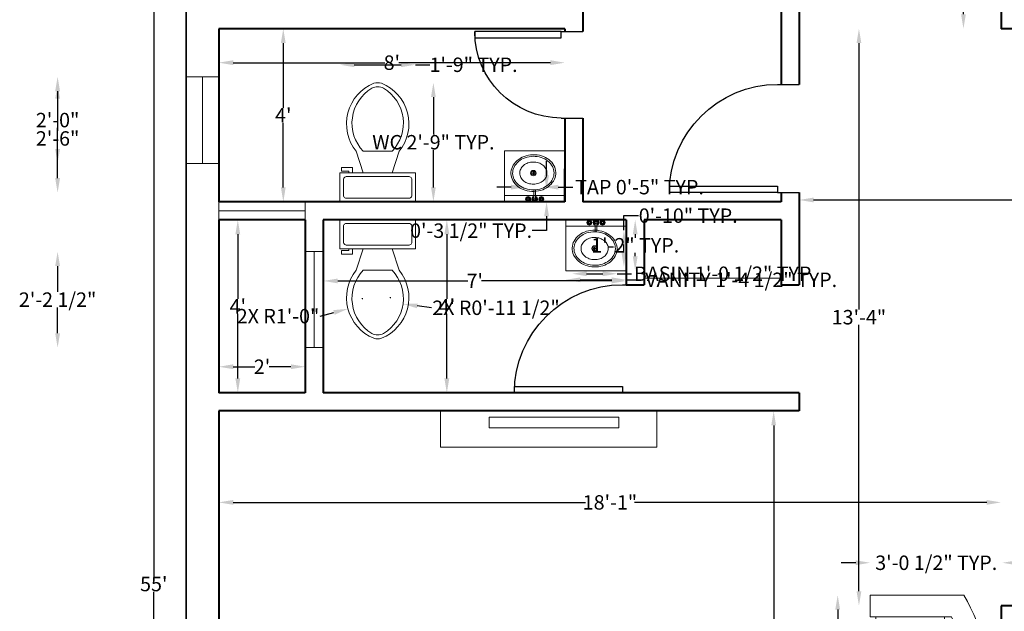
# Model space of a CAD drawing. Units: inches. Extents: x -46 to 447, y -42 to 702.
# Tile 4 of 7: x -46 to 227, y 322 to 487. Entities that reach past the tile are written whole.
import ezdxf

# ---------------------------------------------------------------- set-up
doc = ezdxf.new("R2010")
doc.units = ezdxf.units.IN
doc.header["$PDMODE"] = 3
for name, color, linetype, lineweight in [('A-ANNO-DIMS', 2, 'Continuous', 13), ('A-DOOR', 3, 'Continuous', 25), ('A-FLOR-CASE', 32, 'Continuous', 18), ('A-FLOR-FIXT', 9, 'Continuous', 20), ('A-FURN', 8, 'Continuous', 18), ('A-GLAZ', 4, 'Continuous', 18), ('A-WALL', 7, 'Continuous', 40), ('L-WALL', 7, 'Continuous', 35)]:
    doc.layers.add(name, color=color, linetype=linetype, lineweight=lineweight)
doc.styles.get("Standard").update_dxf_attribs({"font": 'arial.ttf'})
doc.dimstyles.get("Standard").update_dxf_attribs({"dimtxt": 4, "dimasz": 4, "dimexe": 0.18, "dimexo": 0.0625, "dimgap": 0.09, "dimtad": 0, "dimtih": 1, "dimtoh": 1, "dimdec": 0, "dimzin": 0, "dimdsep": 46, "dimlunit": 3, "dimtxsty": 'Standard', "dimcen": 0.09, "dimse1": 1, "dimse2": 1, "dimadec": 0, "dimazin": 0, "dimtfac": 1, "dimtdec": 0, "dimtofl": 0, "dimtmove": 0, "dimatfit": 3, "dimfxl": 1, "dimtolj": 1, "dimtzin": 0, "dimarcsym": 0})

# ---------------------------------------------------------------- blocks, each defined once
blk = doc.blocks.new('*U3')
for p, q in [((-30, 0), (-30, -6)), ((0, 0), (0, -6))]:
    blk.add_line(p, q)
blk.add_lwpolyline([(0, 0), (0, 30), (-1.75, 30), (-1.75, 0)], close=True)
blk.add_arc((0, 0), 30, 90, 180)
blk = doc.blocks.new('*U4')
for p, q in [((0, 0), (0, -6)), ((24, 0), (24, -6))]:
    blk.add_line(p, q)
blk.add_lwpolyline([(0, 0), (0, 24), (1.75, 24), (1.75, 0)], close=True)
blk.add_arc((0, 0), 24, 0, 90)
blk = doc.blocks.new('Faucet - Bathroom top')
for p, q in [((-4.107, 0.125), (-4.375, 0.125)), ((-3.75, 0.4788), (-3.75, 0.75)), ((-3.5, 0.482), (-3.5, 0.75)), ((-3.1461, 0.125), (-2.875, 0.125)), ((3.143, 0.125), (2.875, 0.125)), ((3.5, 0.4788), (3.5, 0.75)), ((3.75, 0.482), (3.75, 0.75)), ((4.1039, 0.125), (4.375, 0.125)), ((-4.1039, -0.125), (-4.375, -0.125)), ((-3.75, -0.4821), (-3.75, -0.75)), ((-3.5, -0.4789), (-3.5, -0.75)), ((-3.143, -0.125), (-2.875, -0.125)), ((-0.5, -0.8639), (-0.5, -4.5)), ((0.5, -4.5), (0.5, -0.8631)), ((3.1461, -0.125), (2.875, -0.125)), ((3.5, -0.4821), (3.5, -0.75)), ((3.75, -0.4789), (3.75, -0.75)), ((4.107, -0.125), (4.375, -0.125))]:
    blk.add_line(p, q)
for centre, radius in [((-3.625, 0), 1.375), ((-4.625, 0), 0.2795), ((-3.625, 0), 0.5), ((-3.625, 1), 0.2795), ((-2.625, 0), 0.2795), ((0, 0), 0.5), ((3.625, 0), 1.375), ((2.625, 0), 0.2795), ((3.625, 0), 0.5), ((3.625, 1), 0.2795), ((4.625, 0), 0.2795), ((-3.625, -1), 0.2795), ((3.625, -1), 0.2795)]:
    blk.add_circle(centre, radius)
for centre, radius, start, end in [((-3.625, 0), 1, 105.2407, 164.2093), ((-3.625, 0), 1, 16.44125, 74.07887), ((0, 0), 1.5, 289.6514, 250.3603), ((0, 0), 1, 300.3431, 239.7554), ((3.625, 0), 1, 106.12, 164.0884), ((3.625, 0), 1, 16.23422, 73.90469), ((-3.625, 0), 1, 196.2342, 253.9047), ((-3.625, 0), 1, 286.12, 344.0884), ((0, -4.5), 0.5, 180, 0), ((3.625, 0), 1, 196.4413, 254.0789), ((3.625, 0), 1, 285.2407, 344.2093)]:
    blk.add_arc(centre, radius, start, end)
blk = doc.blocks.new('Sink - Oval top')
for p, q in [((-1, 0), (1, 0)), ((0, 1), (0, -1))]:
    blk.add_line(p, q)
for points in [[(-12.23, 0.39, 0.117634), (-11.46, -3.36, 0.104469), (-8.88, -6.8, 0.090016), (-5.08, -9.07, 0.08192), (-0.32, -10.02, 0.08192), (4.49, -9.38, 0.090016), (8.42, -7.36, 0.104469), (11.22, -4.09, 0.117634), (12.23, -0.39, 0.117634), (11.46, 3.36, 0.104469), (8.88, 6.8, 0.090016), (5.08, 9.07, 0.08192), (0.32, 10.02, 0.08192), (-4.49, 9.38, 0.090016), (-8.42, 7.36, 0.104469), (-11.22, 4.09, 0.117634)], [(-11.29, 0.16, 0.118622), (-10.52, -3.25, 0.104678), (-8.07, -6.36, 0.089562), (-4.54, -8.37, 0.081185), (-0.13, -9.15, 0.081185), (4.3, -8.49, 0.089562), (7.89, -6.58, 0.104678), (10.42, -3.55, 0.118622), (11.29, -0.16, 0.118622), (10.52, 3.25, 0.104678), (8.07, 6.36, 0.089562), (4.54, 8.37, 0.081185), (0.13, 9.15, 0.081185), (-4.3, 8.49, 0.089562), (-7.89, 6.58, 0.104678), (-10.42, 3.55, 0.118622)], [(-7.42, 0.08, 0.118283), (-6.91, -2.17, 0.104607), (-5.29, -4.21, 0.089718), (-2.97, -5.53, 0.081436), (-0.07, -6.04, 0.081436), (2.84, -5.59, 0.089718), (5.2, -4.33, 0.104607), (6.86, -2.32, 0.118283), (7.42, -0.08, 0.118283), (6.91, 2.17, 0.104607), (5.29, 4.21, 0.089718), (2.97, 5.53, 0.081436), (0.07, 6.04, 0.081436), (-2.84, 5.59, 0.089718), (-5.2, 4.33, 0.104607), (-6.86, 2.32, 0.118283)]]:
    blk.add_lwpolyline(points, format="xyb", close=True)
for radius in [1.5, 1]:
    blk.add_circle((0, 0), radius)
blk = doc.blocks.new('Toilet - top')
for p, q in [((9.5, -6), (9.5, -2)), ((-8, -8.5), (-8, -8)), ((-7, -8), (-7, -9.5)), ((-4, -8), (-6, -14)), ((4, -8), (6, -14)), ((-10, -8.5), (-8, -8.5)), ((-10, -9.5), (-10, -8.5)), ((-7, -9.5), (-10, -9.5)), ((4, -14), (-4, -14))]:
    blk.add_line(p, q)
blk.add_lwpolyline([(10.5, -8), (10.5, 0), (-10.5, 0), (-10.5, -8)], close=True)
for points in [[(-9.5, -2), (-9.5, -6)], [(8.5, -1), (-8.5, -1)], [(-8.5, -7), (8.5, -7)]]:
    blk.add_lwpolyline(points)
for centre, radius, start, end in [((-8.62, -1.88), 0.884, 81.8699, 188.1301), ((8.62, -1.88), 0.884, 351.8699, 98.1301), ((-8.62, -6.12), 0.884, 171.8699, 278.1301), ((8.62, -6.12), 0.884, 261.8699, 8.1301), ((3.52, -21.58), 12.17, 141.4691, 247.9714), ((4.2, -21.82), 11.33, 136.3677, 238.9468), ((-3.52, -21.58), 12.17, 292.0284, 38.5307), ((-4.2, -21.82), 11.33, 301.053, 43.6321), ((0, -27.88), 4, 245.7318, 294.2682), ((0, -29), 4, 254.8605, 285.1395)]:
    blk.add_arc(centre, radius, start, end)
blk = doc.blocks.new('Sofa - Roundback Loveseat 5 ft.')
for p, q in [((0, -32.44198), (0, -5.99998)), ((-24, -33.99998), (-24, -11.46958)), ((-23.9998, -13.38178), (23.99986, -13.38178)), ((24.00004, -33.99998), (24.00004, -11.46958)), ((-24, -32.44198), (24.00004, -32.44198))]:
    blk.add_line(p, q)
for points in [[(-24, -33.99998), (-30, -33.99998), (-30, -7.99998)], [(30.00004, -7.99998), (30.00004, -33.99998), (24.00004, -33.99998)]]:
    blk.add_lwpolyline(points)
for centre, radius, start, end in [((0, -60.24998), 60.24998, 60.13715, 119.8628), ((0, -61.38438), 55.38444, 64.32083, 115.6792)]:
    blk.add_arc(centre, radius, start, end)
blk = doc.blocks.new('*D50')
at = {"layer": 'A-ANNO-DIMS', "color": 0, "lineweight": -2, "transparency": 16777216}
for p, q in [((-9.03, 656), (-9.03, 332.12)), ((-9.03, 4), (-9.03, 327.88))]:
    blk.add_line(p, q, dxfattribs=at)
at = {"layer": 'A-ANNO-DIMS', "color": 0, "transparency": 16777216}
for points in [[(-9.7, 656), (-8.36, 656), (-9.03, 660)], [(-9.7, 4), (-8.36, 4), (-9.03, 0)]]:
    blk.add_solid(points, dxfattribs=at)
at = {"layer": 'Defpoints', "color": 0, "transparency": 16777216}
for p in [(0, 660), (0, 0), (-9.03, 0)]:
    blk.add_point(p, dxfattribs=at)
at = {"layer": 'A-ANNO-DIMS', "color": 0, "transparency": 16777216, "insert": (-9.03, 330), "char_height": 4, "attachment_point": 5}
blk.add_mtext("\\A1;55'", dxfattribs=at)
blk = doc.blocks.new('*D61')
at = {"layer": 'A-ANNO-DIMS', "color": 0, "lineweight": -2, "transparency": 16777216}
for p, q in [((174, 436.51), (250.67, 436.51)), ((344, 436.51), (267.33, 436.51))]:
    blk.add_line(p, q, dxfattribs=at)
at = {"layer": 'A-ANNO-DIMS', "color": 0, "transparency": 16777216}
for points in [[(174, 437.18), (174, 435.84), (170, 436.51)], [(344, 437.18), (344, 435.84), (348, 436.51)]]:
    blk.add_solid(points, dxfattribs=at)
at = {"layer": 'Defpoints', "color": 0, "transparency": 16777216}
for p in [(170, 468.57), (348, 468.57), (348, 436.51)]:
    blk.add_point(p, dxfattribs=at)
at = {"layer": 'A-ANNO-DIMS', "color": 0, "transparency": 16777216, "insert": (259, 436.51), "char_height": 4, "attachment_point": 5}
blk.add_mtext('\\A1;14\'-10"', dxfattribs=at)
blk = doc.blocks.new('*D62')
at = {"layer": 'A-ANNO-DIMS', "color": 0, "lineweight": -2, "transparency": 16777216}
for p, q in [((186.57, 480), (186.57, 406.13)), ((186.57, 328), (186.57, 401.87))]:
    blk.add_line(p, q, dxfattribs=at)
at = {"layer": 'A-ANNO-DIMS', "color": 0, "transparency": 16777216}
for points in [[(185.91, 480), (187.24, 480), (186.57, 484)], [(185.91, 328), (187.24, 328), (186.57, 324)]]:
    blk.add_solid(points, dxfattribs=at)
at = {"layer": 'Defpoints', "color": 0, "transparency": 16777216}
for p in [(312.89, 484), (186.57, 324), (312.89, 324)]:
    blk.add_point(p, dxfattribs=at)
at = {"layer": 'A-ANNO-DIMS', "color": 0, "transparency": 16777216, "insert": (186.57, 404), "char_height": 4, "attachment_point": 5}
blk.add_mtext('\\A1;13\'-4"', dxfattribs=at)
blk = doc.blocks.new('*D63')
at = {"layer": 'A-ANNO-DIMS', "color": 0, "lineweight": -2, "transparency": 16777216}
for p, q in [((13, 352.64), (110.73, 352.64)), ((222, 352.64), (124.27, 352.64))]:
    blk.add_line(p, q, dxfattribs=at)
at = {"layer": 'A-ANNO-DIMS', "color": 0, "transparency": 16777216}
for points in [[(13, 353.31), (13, 351.98), (9, 352.64)], [(222, 353.31), (222, 351.98), (226, 352.64)]]:
    blk.add_solid(points, dxfattribs=at)
at = {"layer": 'Defpoints', "color": 0, "transparency": 16777216}
for p in [(9, 352.64), (9, 324), (226, 324)]:
    blk.add_point(p, dxfattribs=at)
at = {"layer": 'A-ANNO-DIMS', "color": 0, "transparency": 16777216, "insert": (117.5, 352.64), "char_height": 4, "attachment_point": 5}
blk.add_mtext('\\A1;18\'-1"', dxfattribs=at)
blk = doc.blocks.new('*D64')
at = {"layer": 'A-ANNO-DIMS', "color": 0, "lineweight": -2, "transparency": 16777216}
for p, q in [((162.92, 374), (162.92, 296.1)), ((162.92, 214), (162.92, 291.9))]:
    blk.add_line(p, q, dxfattribs=at)
at = {"layer": 'A-ANNO-DIMS', "color": 0, "transparency": 16777216}
for points in [[(162.25, 374), (163.58, 374), (162.92, 378)], [(162.25, 214), (163.58, 214), (162.92, 210)]]:
    blk.add_solid(points, dxfattribs=at)
at = {"layer": 'Defpoints', "color": 0, "transparency": 16777216}
for p in [(9, 378), (9, 210), (162.92, 210)]:
    blk.add_point(p, dxfattribs=at)
at = {"layer": 'A-ANNO-DIMS', "color": 0, "transparency": 16777216, "insert": (162.92, 294), "char_height": 4, "attachment_point": 5}
blk.add_mtext("\\A1;14'", dxfattribs=at)
blk = doc.blocks.new('*D65')
at = {"layer": 'A-ANNO-DIMS', "color": 0, "lineweight": -2, "transparency": 16777216}
for p, q in [((14.28, 427), (14.28, 409.09)), ((14.28, 387), (14.28, 404.91))]:
    blk.add_line(p, q, dxfattribs=at)
at = {"layer": 'A-ANNO-DIMS', "color": 0, "transparency": 16777216}
for points in [[(13.61, 427), (14.95, 427), (14.28, 431)], [(13.61, 387), (14.95, 387), (14.28, 383)]]:
    blk.add_solid(points, dxfattribs=at)
at = {"layer": 'Defpoints', "color": 0, "transparency": 16777216}
for p in [(9, 431), (9, 383), (14.28, 383)]:
    blk.add_point(p, dxfattribs=at)
at = {"layer": 'A-ANNO-DIMS', "color": 0, "transparency": 16777216, "insert": (14.28, 407), "char_height": 4, "attachment_point": 5}
blk.add_mtext("\\A1;4'", dxfattribs=at)
blk = doc.blocks.new('*D66')
at = {"layer": 'A-ANNO-DIMS', "color": 0, "lineweight": -2, "transparency": 16777216}
for p, q in [((13, 390.26), (19.04, 390.26)), ((29, 390.26), (22.96, 390.26))]:
    blk.add_line(p, q, dxfattribs=at)
at = {"layer": 'A-ANNO-DIMS', "color": 0, "transparency": 16777216}
for points in [[(13, 390.93), (13, 389.6), (9, 390.26)], [(29, 390.93), (29, 389.6), (33, 390.26)]]:
    blk.add_solid(points, dxfattribs=at)
at = {"layer": 'Defpoints', "color": 0, "transparency": 16777216}
for p in [(9, 390.26), (9, 383), (33, 383)]:
    blk.add_point(p, dxfattribs=at)
at = {"layer": 'A-ANNO-DIMS', "color": 0, "transparency": 16777216, "insert": (21, 390.26), "char_height": 4, "attachment_point": 5}
blk.add_mtext("\\A1;2'", dxfattribs=at)
blk = doc.blocks.new('*D67')
at = {"layer": 'A-ANNO-DIMS', "color": 0, "lineweight": -2, "transparency": 16777216}
for p, q in [((42, 414.06), (78.09, 414.06)), ((118, 414.06), (81.91, 414.06))]:
    blk.add_line(p, q, dxfattribs=at)
at = {"layer": 'A-ANNO-DIMS', "color": 0, "transparency": 16777216}
for points in [[(42, 414.72), (42, 413.39), (38, 414.06)], [(118, 414.72), (118, 413.39), (122, 414.06)]]:
    blk.add_solid(points, dxfattribs=at)
at = {"layer": 'Defpoints', "color": 0, "transparency": 16777216}
for p in [(38, 431), (122, 431), (38, 414.06)]:
    blk.add_point(p, dxfattribs=at)
at = {"layer": 'A-ANNO-DIMS', "color": 0, "transparency": 16777216, "insert": (80, 414.06), "char_height": 4, "attachment_point": 5}
blk.add_mtext("\\A1;7'", dxfattribs=at)
blk = doc.blocks.new('*D68')
at = {"layer": 'A-ANNO-DIMS', "color": 0, "lineweight": -2, "transparency": 16777216}
for p, q in [((72.26, 427), (72.26, 409.09)), ((72.26, 387), (72.26, 404.91))]:
    blk.add_line(p, q, dxfattribs=at)
at = {"layer": 'A-ANNO-DIMS', "color": 0, "transparency": 16777216}
for points in [[(71.59, 427), (72.93, 427), (72.26, 431)], [(71.59, 387), (72.93, 387), (72.26, 383)]]:
    blk.add_solid(points, dxfattribs=at)
at = {"layer": 'Defpoints', "color": 0, "transparency": 16777216}
for p in [(38, 431), (38, 383), (72.26, 383)]:
    blk.add_point(p, dxfattribs=at)
at = {"layer": 'A-ANNO-DIMS', "color": 0, "transparency": 16777216, "insert": (72.26, 407), "char_height": 4, "attachment_point": 5}
blk.add_mtext("\\A1;4'", dxfattribs=at)
blk = doc.blocks.new('*D69')
at = {"layer": 'A-ANNO-DIMS', "color": 0, "lineweight": -2, "transparency": 16777216}
for p, q in [((215.55, 546), (215.55, 519.13)), ((215.55, 488), (215.55, 514.87))]:
    blk.add_line(p, q, dxfattribs=at)
at = {"layer": 'A-ANNO-DIMS', "color": 0, "transparency": 16777216}
for points in [[(214.89, 546), (216.22, 546), (215.55, 550)], [(214.89, 488), (216.22, 488), (215.55, 484)]]:
    blk.add_solid(points, dxfattribs=at)
at = {"layer": 'Defpoints', "color": 0, "transparency": 16777216}
for p in [(226, 550), (215.55, 484), (226, 484)]:
    blk.add_point(p, dxfattribs=at)
at = {"layer": 'A-ANNO-DIMS', "color": 0, "transparency": 16777216, "insert": (215.55, 517), "char_height": 4, "attachment_point": 5}
blk.add_mtext('\\A1;5\'-6"', dxfattribs=at)
blk = doc.blocks.new('*D75')
at = {"layer": 'A-ANNO-DIMS', "color": 0, "lineweight": -2, "transparency": 16777216}
for p, q in [((13, 474.58), (55.07, 474.58)), ((101, 474.58), (58.93, 474.58))]:
    blk.add_line(p, q, dxfattribs=at)
at = {"layer": 'A-ANNO-DIMS', "color": 0, "transparency": 16777216}
for points in [[(13, 475.25), (13, 473.92), (9, 474.58)], [(101, 475.25), (101, 473.92), (105, 474.58)]]:
    blk.add_solid(points, dxfattribs=at)
at = {"layer": 'Defpoints', "color": 0, "transparency": 16777216}
for p in [(9, 484), (105, 484), (9, 474.58)]:
    blk.add_point(p, dxfattribs=at)
at = {"layer": 'A-ANNO-DIMS', "color": 0, "transparency": 16777216, "insert": (57, 474.58), "char_height": 4, "attachment_point": 5}
blk.add_mtext("\\A1;8'", dxfattribs=at)
blk = doc.blocks.new('*D76')
at = {"layer": 'A-ANNO-DIMS', "color": 0, "lineweight": -2, "transparency": 16777216}
for p, q in [((26.9, 480), (26.9, 462.09)), ((26.9, 440), (26.9, 457.91))]:
    blk.add_line(p, q, dxfattribs=at)
at = {"layer": 'A-ANNO-DIMS', "color": 0, "transparency": 16777216}
for points in [[(26.23, 480), (27.56, 480), (26.9, 484)], [(26.23, 440), (27.56, 440), (26.9, 436)]]:
    blk.add_solid(points, dxfattribs=at)
at = {"layer": 'Defpoints', "color": 0, "transparency": 16777216}
for p in [(9, 484), (9, 436), (26.9, 436)]:
    blk.add_point(p, dxfattribs=at)
at = {"layer": 'A-ANNO-DIMS', "color": 0, "transparency": 16777216, "insert": (26.9, 460), "char_height": 4, "attachment_point": 5}
blk.add_mtext("\\A1;4'", dxfattribs=at)
blk = doc.blocks.new('VANITY-TOP')
for points in [[(0, -1.75), (16.74, -1.75), (16.74, 0), (0, 0)], [(0, -1.75), (16.74, -1.75), (16.74, -14.12), (0, -14.12)]]:
    blk.add_lwpolyline(points, close=True)
blk = doc.blocks.new('*D94')
at = {"layer": 'A-ANNO-DIMS', "color": 0, "lineweight": -2, "transparency": 16777216}
for p, q in [((90.09, 440.07), (86.09, 440.07)), ((103.17, 440.07), (107.17, 440.07))]:
    blk.add_line(p, q, dxfattribs=at)
at = {"layer": 'A-ANNO-DIMS', "color": 0, "transparency": 16777216}
for points in [[(90.09, 440.74), (90.09, 439.4), (94.09, 440.07)], [(103.17, 440.74), (103.17, 439.4), (99.17, 440.07)]]:
    blk.add_solid(points, dxfattribs=at)
at = {"layer": 'Defpoints', "color": 0, "transparency": 16777216}
for p in [(99.17, 440.07), (94.09, 439.31), (99.17, 439.31)]:
    blk.add_point(p, dxfattribs=at)
at = {"layer": 'A-ANNO-DIMS', "color": 0, "transparency": 16777216, "insert": (125.71, 440.07), "char_height": 4, "attachment_point": 5}
blk.add_mtext('\\A1;TAP 0\'-5" TYP.', dxfattribs=at)
blk = doc.blocks.new('*D95')
at = {"layer": 'A-ANNO-DIMS', "color": 0, "lineweight": -2, "transparency": 16777216}
for p, q in [((99.93, 443.31), (99.93, 447.31)), ((99.93, 432), (99.93, 428)), ((99.93, 428), (95.93, 428))]:
    blk.add_line(p, q, dxfattribs=at)
at = {"layer": 'A-ANNO-DIMS', "color": 0, "transparency": 16777216}
for points in [[(99.27, 443.31), (100.6, 443.31), (99.93, 439.31)], [(99.27, 432), (100.6, 432), (99.93, 436)]]:
    blk.add_solid(points, dxfattribs=at)
at = {"layer": 'Defpoints', "color": 0, "transparency": 16777216}
for p in [(99.17, 439.31), (99.17, 436), (99.93, 436)]:
    blk.add_point(p, dxfattribs=at)
at = {"layer": 'A-ANNO-DIMS', "color": 0, "transparency": 16777216, "insert": (78.99, 428), "char_height": 4, "attachment_point": 5}
blk.add_mtext('\\A1;0\'-3 1/2" TYP.', dxfattribs=at)
blk = doc.blocks.new('*D96')
at = {"layer": 'A-ANNO-DIMS', "color": 0, "lineweight": -2, "transparency": 16777216}
for p, q in [((111.02, 416.05), (115.51, 416.05)), ((119.51, 416.05), (123.51, 416.05))]:
    blk.add_line(p, q, dxfattribs=at)
at = {"layer": 'A-ANNO-DIMS', "color": 0, "transparency": 16777216}
for points in [[(111.02, 416.72), (111.02, 415.38), (107.02, 416.05)], [(115.51, 416.72), (115.51, 415.38), (119.51, 416.05)]]:
    blk.add_solid(points, dxfattribs=at)
at = {"layer": 'Defpoints', "color": 0, "transparency": 16777216}
for p in [(107.02, 417.92), (119.51, 417.92), (119.51, 416.05)]:
    blk.add_point(p, dxfattribs=at)
at = {"layer": 'A-ANNO-DIMS', "color": 0, "transparency": 16777216, "insert": (149.52, 416.05), "char_height": 4, "attachment_point": 5}
blk.add_mtext('\\A1;BASIN 1\'-0 1/2" TYP.', dxfattribs=at)
blk = doc.blocks.new('*D97')
at = {"layer": 'A-ANNO-DIMS', "color": 0, "lineweight": -2, "transparency": 16777216}
for p, q in [((121.38, 428.16), (121.38, 432.16)), ((121.38, 432.16), (125.38, 432.16)), ((121.38, 421.92), (121.38, 424.16))]:
    blk.add_line(p, q, dxfattribs=at)
at = {"layer": 'A-ANNO-DIMS', "color": 0, "transparency": 16777216}
for points in [[(120.71, 424.16), (122.04, 424.16), (121.38, 428.16)], [(120.71, 421.92), (122.04, 421.92), (121.38, 417.92)]]:
    blk.add_solid(points, dxfattribs=at)
at = {"layer": 'Defpoints', "color": 0, "transparency": 16777216}
for p in [(119.51, 428.16), (121.38, 428.16), (119.51, 417.92)]:
    blk.add_point(p, dxfattribs=at)
at = {"layer": 'A-ANNO-DIMS', "color": 0, "transparency": 16777216, "insert": (139.21, 432.16), "char_height": 4, "attachment_point": 5}
blk.add_mtext('\\A1;0\'-10" TYP.', dxfattribs=at)
blk = doc.blocks.new('*D98')
at = {"layer": 'A-ANNO-DIMS', "color": 0, "lineweight": -2, "transparency": 16777216}
for p, q in [((68.53, 465.05), (68.53, 454.68)), ((68.53, 440), (68.53, 450.36))]:
    blk.add_line(p, q, dxfattribs=at)
at = {"layer": 'A-ANNO-DIMS', "color": 0, "transparency": 16777216}
for points in [[(67.87, 465.05), (69.2, 465.05), (68.53, 469.05)], [(67.87, 440), (69.2, 440), (68.53, 436)]]:
    blk.add_solid(points, dxfattribs=at)
at = {"layer": 'Defpoints', "color": 0, "transparency": 16777216}
for p in [(63.58, 469.05), (63.58, 436), (68.53, 436)]:
    blk.add_point(p, dxfattribs=at)
at = {"layer": 'A-ANNO-DIMS', "color": 0, "transparency": 16777216, "insert": (68.53, 452.52), "char_height": 4, "attachment_point": 5}
blk.add_mtext('\\A1;WC 2\'-9" TYP.', dxfattribs=at)
blk = doc.blocks.new('*D99')
at = {"layer": 'A-ANNO-DIMS', "color": 0, "lineweight": -2, "transparency": 16777216}
for p, q in [((46.58, 474), (59.58, 474)), ((63.58, 474), (67.58, 474))]:
    blk.add_line(p, q, dxfattribs=at)
at = {"layer": 'A-ANNO-DIMS', "color": 0, "transparency": 16777216}
for points in [[(46.58, 474.67), (46.58, 473.34), (42.58, 474)], [(59.58, 474.67), (59.58, 473.34), (63.58, 474)]]:
    blk.add_solid(points, dxfattribs=at)
at = {"layer": 'Defpoints', "color": 0, "transparency": 16777216}
for p in [(63.58, 474), (42.58, 469.05), (63.58, 469.05)]:
    blk.add_point(p, dxfattribs=at)
at = {"layer": 'A-ANNO-DIMS', "color": 0, "transparency": 16777216, "insert": (79.67, 474), "char_height": 4, "attachment_point": 5}
blk.add_mtext('\\A1;1\'-9" TYP.', dxfattribs=at)
blk = doc.blocks.new('*D100')
at = {"layer": 'A-ANNO-DIMS', "color": 0, "lineweight": -2, "transparency": 16777216}
for p, q in [((109.26, 414.37), (118, 414.37)), ((122, 414.37), (126, 414.37))]:
    blk.add_line(p, q, dxfattribs=at)
at = {"layer": 'A-ANNO-DIMS', "color": 0, "transparency": 16777216}
for points in [[(109.26, 415.03), (109.26, 413.7), (105.26, 414.37)], [(118, 415.03), (118, 413.7), (122, 414.37)]]:
    blk.add_solid(points, dxfattribs=at)
at = {"layer": 'Defpoints', "color": 0, "transparency": 16777216}
for p in [(105.26, 416.88), (122, 416.88), (122, 414.37)]:
    blk.add_point(p, dxfattribs=at)
at = {"layer": 'A-ANNO-DIMS', "color": 0, "transparency": 16777216, "insert": (153.91, 414.37), "char_height": 4, "attachment_point": 5}
blk.add_mtext('\\A1;VANITY 1\'-4 1/2" TYP.', dxfattribs=at)
blk = doc.blocks.new('*D101')
at = {"layer": 'A-ANNO-DIMS', "color": 0, "lineweight": -2, "transparency": 16777216}
for p, q in [((124.51, 427), (124.51, 426.04)), ((124.51, 420.88), (124.51, 421.84))]:
    blk.add_line(p, q, dxfattribs=at)
at = {"layer": 'A-ANNO-DIMS', "color": 0, "transparency": 16777216}
for points in [[(123.84, 427), (125.18, 427), (124.51, 431)], [(123.84, 420.88), (125.18, 420.88), (124.51, 416.88)]]:
    blk.add_solid(points, dxfattribs=at)
at = {"layer": 'Defpoints', "color": 0, "transparency": 16777216}
for p in [(122, 431), (124.51, 431), (122, 416.88)]:
    blk.add_point(p, dxfattribs=at)
at = {"layer": 'A-ANNO-DIMS', "color": 0, "transparency": 16777216, "insert": (124.51, 423.94), "char_height": 4, "attachment_point": 5}
blk.add_mtext('\\A1;1\'-2" TYP.', dxfattribs=at)
blk = doc.blocks.new('*D106')
at = {"layer": 'A-ANNO-DIMS', "color": 0, "lineweight": -2, "transparency": 16777216}
for p, q in [((180.68, 322.9), (180.68, 299.06)), ((180.68, 270.9), (180.68, 294.74))]:
    blk.add_line(p, q, dxfattribs=at)
at = {"layer": 'A-ANNO-DIMS', "color": 0, "transparency": 16777216}
for points in [[(180.01, 322.9), (181.34, 322.9), (180.68, 326.9)], [(180.01, 270.9), (181.34, 270.9), (180.68, 266.9)]]:
    blk.add_solid(points, dxfattribs=at)
at = {"layer": 'Defpoints', "color": 0, "transparency": 16777216}
for p in [(180.68, 326.9), (189.68, 326.9), (189.68, 266.9)]:
    blk.add_point(p, dxfattribs=at)
at = {"layer": 'A-ANNO-DIMS', "color": 0, "transparency": 16777216, "insert": (180.68, 296.9), "char_height": 4, "attachment_point": 5}
blk.add_mtext('\\A1;LOVESEAT 5\'-0" TYP.', dxfattribs=at)
blk = doc.blocks.new('*D107')
at = {"layer": 'A-ANNO-DIMS', "color": 0, "lineweight": -2, "transparency": 16777216}
for p, q in [((185.68, 335.9), (181.68, 335.9)), ((230.34, 335.9), (234.34, 335.9))]:
    blk.add_line(p, q, dxfattribs=at)
at = {"layer": 'A-ANNO-DIMS', "color": 0, "transparency": 16777216}
for points in [[(185.68, 336.57), (185.68, 335.24), (189.68, 335.9)], [(230.34, 336.57), (230.34, 335.24), (226.34, 335.9)]]:
    blk.add_solid(points, dxfattribs=at)
at = {"layer": 'Defpoints', "color": 0, "transparency": 16777216}
for p in [(226.34, 335.9), (189.68, 326.9), (226.34, 326.9)]:
    blk.add_point(p, dxfattribs=at)
at = {"layer": 'A-ANNO-DIMS', "color": 0, "transparency": 16777216, "insert": (208.01, 335.9), "char_height": 4, "attachment_point": 5}
blk.add_mtext('\\A1;3\'-0 1/2" TYP.', dxfattribs=at)
blk = doc.blocks.new('*D125')
at = {"layer": 'A-ANNO-DIMS', "color": 0, "lineweight": -2, "transparency": 16777216}
for p, q in [((-35.7, 464.57), (-35.7, 455.71)), ((-35.7, 442.57), (-35.7, 451.44))]:
    blk.add_line(p, q, dxfattribs=at)
at = {"layer": 'A-ANNO-DIMS', "color": 0, "transparency": 16777216}
for points in [[(-36.37, 464.57), (-35.03, 464.57), (-35.7, 468.57)], [(-36.37, 442.57), (-35.03, 442.57), (-35.7, 438.57)]]:
    blk.add_solid(points, dxfattribs=at)
at = {"layer": 'Defpoints', "color": 0, "transparency": 16777216}
for p in [(-35.7, 468.57), (165, 468.57), (165, 438.57)]:
    blk.add_point(p, dxfattribs=at)
at = {"layer": 'A-ANNO-DIMS', "color": 0, "transparency": 16777216, "insert": (-35.7, 453.57), "char_height": 4, "attachment_point": 5}
blk.add_mtext('\\A1;2\'-6"', dxfattribs=at)
blk = doc.blocks.new('*D126')
at = {"layer": 'A-ANNO-DIMS', "color": 0, "lineweight": -2, "transparency": 16777216}
for p, q in [((431.7, 409), (431.7, 400.13)), ((431.7, 387), (431.7, 395.87))]:
    blk.add_line(p, q, dxfattribs=at)
at = {"layer": 'A-ANNO-DIMS', "color": 0, "transparency": 16777216}
for points in [[(431.03, 409), (432.37, 409), (431.7, 413)], [(431.03, 387), (432.37, 387), (431.7, 383)]]:
    blk.add_solid(points, dxfattribs=at)
at = {"layer": 'Defpoints', "color": 0, "transparency": 16777216}
for p in [(122, 413), (431.7, 413), (122.75, 383)]:
    blk.add_point(p, dxfattribs=at)
at = {"layer": 'A-ANNO-DIMS', "color": 0, "transparency": 16777216, "insert": (431.7, 398), "char_height": 4, "attachment_point": 5}
blk.add_mtext('\\A1;2\'-6"', dxfattribs=at)
blk = doc.blocks.new('*D127')
at = {"layer": 'A-ANNO-DIMS', "color": 0, "lineweight": -2, "transparency": 16777216}
for p, q in [((431.7, 479.23), (431.7, 473.36)), ((431.7, 463.23), (431.7, 469.1))]:
    blk.add_line(p, q, dxfattribs=at)
at = {"layer": 'A-ANNO-DIMS', "color": 0, "transparency": 16777216}
for points in [[(431.03, 479.23), (432.37, 479.23), (431.7, 483.23)], [(431.03, 463.23), (432.37, 463.23), (431.7, 459.23)]]:
    blk.add_solid(points, dxfattribs=at)
at = {"layer": 'Defpoints', "color": 0, "transparency": 16777216}
for p in [(105, 483.23), (431.7, 483.23), (105, 459.23)]:
    blk.add_point(p, dxfattribs=at)
at = {"layer": 'A-ANNO-DIMS', "color": 0, "transparency": 16777216, "insert": (431.7, 471.23), "char_height": 4, "attachment_point": 5}
blk.add_mtext('\\A1;2\'-0"', dxfattribs=at)
blk = doc.blocks.new('*D128')
at = {"layer": 'A-ANNO-DIMS', "color": 0, "lineweight": -2, "transparency": 16777216}
for p, q in [((-35.7, 466.66), (-35.7, 460.79)), ((-35.7, 450.66), (-35.7, 456.52))]:
    blk.add_line(p, q, dxfattribs=at)
at = {"layer": 'A-ANNO-DIMS', "color": 0, "transparency": 16777216}
for points in [[(-36.37, 466.66), (-35.03, 466.66), (-35.7, 470.66)], [(-36.37, 450.66), (-35.03, 450.66), (-35.7, 446.66)]]:
    blk.add_solid(points, dxfattribs=at)
at = {"layer": 'Defpoints', "color": 0, "transparency": 16777216}
for p in [(-35.7, 470.66), (0, 470.66), (0, 446.66)]:
    blk.add_point(p, dxfattribs=at)
at = {"layer": 'A-ANNO-DIMS', "color": 0, "transparency": 16777216, "insert": (-35.7, 458.66), "char_height": 4, "attachment_point": 5}
blk.add_mtext('\\A1;2\'-0"', dxfattribs=at)
blk = doc.blocks.new('*D129')
at = {"layer": 'A-ANNO-DIMS', "color": 0, "lineweight": -2, "transparency": 16777216}
for p, q in [((29, -35.7), (25, -35.7)), ((42, -35.7), (46, -35.7))]:
    blk.add_line(p, q, dxfattribs=at)
at = {"layer": 'A-ANNO-DIMS', "color": 0, "transparency": 16777216}
for points in [[(29, -35.03), (29, -36.37), (33, -35.7)], [(42, -35.03), (42, -36.37), (38, -35.7)]]:
    blk.add_solid(points, dxfattribs=at)
at = {"layer": 'Defpoints', "color": 0, "transparency": 16777216}
for p in [(33, 383), (38, 383), (38, -35.7)]:
    blk.add_point(p, dxfattribs=at)
at = {"layer": 'A-ANNO-DIMS', "color": 0, "transparency": 16777216, "insert": (51.41, -35.7), "char_height": 4, "attachment_point": 5}
blk.add_mtext('\\A1;0\'-5"', dxfattribs=at)
blk = doc.blocks.new('*D130')
at = {"layer": 'A-ANNO-DIMS', "color": 0, "lineweight": -2, "transparency": 16777216}
for p, q in [((0, 695.7), (-4, 695.7)), ((5, 695.7), (4, 695.7))]:
    blk.add_line(p, q, dxfattribs=at)
at = {"layer": 'A-ANNO-DIMS', "color": 0, "transparency": 16777216}
for points in [[(4, 696.37), (4, 695.03), (0, 695.7)], [(5, 696.37), (5, 695.03), (9, 695.7)]]:
    blk.add_solid(points, dxfattribs=at)
at = {"layer": 'Defpoints', "color": 0, "transparency": 16777216}
for p in [(0, 695.7), (0, 446.66), (9, 446.66)]:
    blk.add_point(p, dxfattribs=at)
at = {"layer": 'A-ANNO-DIMS', "color": 0, "transparency": 16777216, "insert": (-9.41, 695.7), "char_height": 4, "attachment_point": 5}
blk.add_mtext('\\A1;0\'-9"', dxfattribs=at)
blk = doc.blocks.new('*D138')
at = {"layer": 'A-ANNO-DIMS', "color": 0, "lineweight": -2, "transparency": 16777216}
for p, q in [((-35.7, 418.18), (-35.7, 411.03)), ((-35.7, 399.56), (-35.7, 406.71))]:
    blk.add_line(p, q, dxfattribs=at)
at = {"layer": 'A-ANNO-DIMS', "color": 0, "transparency": 16777216}
for points in [[(-36.37, 418.18), (-35.03, 418.18), (-35.7, 422.18)], [(-36.37, 399.56), (-35.03, 399.56), (-35.7, 395.56)]]:
    blk.add_solid(points, dxfattribs=at)
at = {"layer": 'Defpoints', "color": 0, "transparency": 16777216}
for p in [(-35.7, 422.18), (33, 422.18), (33, 395.56)]:
    blk.add_point(p, dxfattribs=at)
at = {"layer": 'A-ANNO-DIMS', "color": 0, "transparency": 16777216, "insert": (-35.7, 408.87), "char_height": 4, "attachment_point": 5}
blk.add_mtext('\\A1;2\'-2 1/2"', dxfattribs=at)
blk = doc.blocks.new('*D148')
at = {"layer": 'A-ANNO-DIMS', "color": 0, "lineweight": -2, "transparency": 16777216}
for p, q in [((227, 695.7), (223, 695.7)), ((238.24, 695.7), (242.24, 695.7))]:
    blk.add_line(p, q, dxfattribs=at)
at = {"layer": 'A-ANNO-DIMS', "color": 0, "transparency": 16777216}
for points in [[(227, 696.37), (227, 695.03), (231, 695.7)], [(238.24, 696.37), (238.24, 695.03), (234.24, 695.7)]]:
    blk.add_solid(points, dxfattribs=at)
at = {"layer": 'Defpoints', "color": 0, "transparency": 16777216}
for p in [(234.24, 695.7), (231, 319), (234.24, 319)]:
    blk.add_point(p, dxfattribs=at)
at = {"layer": 'A-ANNO-DIMS', "color": 0, "transparency": 16777216, "insert": (247.64, 695.7), "char_height": 4, "attachment_point": 5}
blk.add_mtext('\\A1;0\'-3"', dxfattribs=at)
blk = doc.blocks.new('*D159')
at = {"layer": 'A-ANNO-DIMS', "color": 0, "lineweight": -2, "transparency": 16777216}
for p, q in [((56.51, 409.42), (56.69, 409.42)), ((56.6, 409.33), (56.6, 409.51)), ((37.09, 404.29), (40.96, 405.31))]:
    blk.add_line(p, q, dxfattribs=at)
at = {"layer": 'A-ANNO-DIMS', "color": 0, "transparency": 16777216}
blk.add_solid([(40.79, 405.96), (41.13, 404.67), (44.83, 406.33)], dxfattribs=at)
at = {"layer": 'Defpoints', "color": 0, "transparency": 16777216}
for p in [(56.6, 409.42), (44.83, 406.33)]:
    blk.add_point(p, dxfattribs=at)
at = {"layer": 'A-ANNO-DIMS', "color": 0, "transparency": 16777216, "insert": (25.44, 404.29), "char_height": 4, "attachment_point": 5}
blk.add_mtext('\\A1;2X R1\'-0"', dxfattribs=at)
blk = doc.blocks.new('*D160')
at = {"layer": 'A-ANNO-DIMS', "color": 0, "lineweight": -2, "transparency": 16777216}
for p, q in [((48.79, 409.18), (48.97, 409.18)), ((48.88, 409.09), (48.88, 409.27)), ((68.03, 406.61), (64.07, 407.14))]:
    blk.add_line(p, q, dxfattribs=at)
at = {"layer": 'A-ANNO-DIMS', "color": 0, "transparency": 16777216}
blk.add_solid([(64.16, 407.8), (63.98, 406.48), (60.11, 407.67)], dxfattribs=at)
at = {"layer": 'Defpoints', "color": 0, "transparency": 16777216}
for p in [(48.88, 409.18), (60.11, 407.67)]:
    blk.add_point(p, dxfattribs=at)
at = {"layer": 'A-ANNO-DIMS', "color": 0, "transparency": 16777216, "insert": (85.9, 406.61), "char_height": 4, "attachment_point": 5}
blk.add_mtext('\\A1;2X R0\'-11 1/2"', dxfattribs=at)

msp = doc.modelspace()

# ---------------------------------------------------------------- linework, layer by layer
at = {"layer": 'A-FLOR-CASE'}
msp.add_line((127, 414.83), (165, 414.83), dxfattribs=at)
for points in [[(70.49, 378), (130.49, 378), (130.49, 368), (70.49, 368)], [(83.97, 376.3), (119.97, 376.3), (119.97, 373.3), (83.97, 373.3)]]:
    msp.add_lwpolyline(points, close=True, dxfattribs=at)
at = {"layer": 'A-GLAZ'}
for p, q in [((0, 470.66), (9, 470.66)), ((4.5, 470.66), (4.5, 446.66)), ((0, 446.66), (9, 446.66)), ((9, 436), (9, 431)), ((33, 431), (33, 436)), ((9, 433.5), (33, 433.5)), ((33, 422.18), (38, 422.18)), ((35.5, 422.18), (35.5, 395.56)), ((33, 395.56), (38, 395.56))]:
    msp.add_line(p, q, dxfattribs=at)
at = {"layer": 'A-WALL'}
for p, q in [((165, 651), (165, 468.57)), ((170, 550), (170, 468.57)), ((226, 550), (226, 484)), ((110, 489), (110, 483.23)), ((105, 484), (9, 484)), ((9, 484), (9, 436)), ((105, 484), (105, 483.23)), ((255, 484), (226, 484)), ((105, 459.23), (105, 436)), ((110, 459.23), (110, 436)), ((105, 436), (105, 445.15)), ((165, 438.57), (165, 436)), ((170, 438.57), (170, 413)), ((105, 436), (9, 436)), ((165, 436), (110, 436)), ((9, 431), (9, 383)), ((33, 431), (9, 431)), ((33, 431), (33, 383)), ((38, 431), (38, 383)), ((122, 431), (38, 431)), ((122, 431), (122, 421.85)), ((122, 431), (122, 413)), ((165, 431), (127, 431)), ((127, 431), (127, 413)), ((165, 431), (165, 413)), ((122, 413), (127, 413)), ((165, 413), (170, 413)), ((33, 383), (9, 383)), ((170, 383), (38, 383)), ((170, 383), (170, 378)), ((170, 378), (9, 378)), ((9, 378), (9, 210)), ((226, 324), (226, 210)), ((234.24, 324), (226, 324))]:
    msp.add_line(p, q, dxfattribs=at)
at = {"layer": 'L-WALL'}
msp.add_lwpolyline([(222, 0), (396, 0), (396, 660), (0, 660), (0, 0), (17.93, 0)], dxfattribs=at)

# ---------------------------------------------------------------- block references
at = {"layer": 'A-DOOR', "xscale": -1, "rotation": 90}
for name, p in [('*U4', (104, 483.23)), ('*U3', (164, 438.57)), ('*U3', (121, 383))]:
    msp.add_blockref(name, p, dxfattribs=at)
at = {"layer": 'A-FLOR-CASE', "extrusion": (0, 0, -1), "zscale": -1, "rotation": 180}
msp.add_blockref('VANITY-TOP', (-88.26, 436), dxfattribs=at)
at = {"layer": 'A-FLOR-CASE'}
msp.add_blockref('VANITY-TOP', (105.26, 431), dxfattribs=at)
at = {"layer": 'A-FLOR-FIXT', "xscale": -1, "rotation": 180}
msp.add_blockref('Toilet - top', (53.08, 436), dxfattribs=at)
at = {"layer": 'A-FLOR-FIXT', "xscale": -0.5085474315686545, "yscale": 0.5085474315686545, "zscale": 0.5085474315686545, "rotation": 180}
for name, p in [('Sink - Oval top', (96.26, 443.96)), ('Faucet - Bathroom top', (96.63, 436.76))]:
    msp.add_blockref(name, p, dxfattribs=at)
at = {"layer": 'A-FLOR-FIXT'}
msp.add_blockref('Toilet - top', (53.08, 431), dxfattribs=at)
at = {"layer": 'A-FLOR-FIXT', "xscale": 0.5085474315686545, "yscale": 0.5085474315686545, "zscale": 0.5085474315686545}
for name, p in [('Faucet - Bathroom top', (113.63, 430.24)), ('Sink - Oval top', (113.26, 423.04))]:
    msp.add_blockref(name, p, dxfattribs=at)
at = {"layer": 'A-FURN', "xscale": -1, "rotation": 270}
msp.add_blockref('Sofa - Roundback Loveseat 5 ft.', (223.68, 296.9), dxfattribs=at)

# ---------------------------------------------------------------- dimensions: what is measured, and where the dimension line sits
at = {"layer": 'A-ANNO-DIMS'}
for base, p1, p2, override, picture, middle in [((0, 695.7), (9, 446.66), (0, 446.66), {"dimdec": 1, "dimlfac": 1, "dimrnd": 0, "dimzin": 1, "dimdsep": 46, "dimlunit": 4, "dimfrac": 2}, '*D130', (-9.41, 695.7)), ((234.24, 695.7), (231, 319), (234.24, 319), {"dimdec": 1, "dimlfac": 1, "dimrnd": 0, "dimzin": 1, "dimdsep": 46, "dimlunit": 4, "dimfrac": 2}, '*D148', (247.64, 695.7)), ((9, 474.58), (105, 484), (9, 484), {"dimclrd": 0, "dimclre": 0, "dimclrt": 0}, '*D75', (57, 474.58)), ((348, 436.51), (170, 468.57), (348, 468.57), {"dimclrd": 0, "dimclre": 0, "dimclrt": 0}, '*D61', (259, 436.51)), ((38, 414.06), (122, 431), (38, 431), {"dimclrd": 0, "dimclre": 0, "dimclrt": 0}, '*D67', (80, 414.06)), ((9, 390.26), (33, 383), (9, 383), {"dimclrd": 0, "dimclre": 0, "dimclrt": 0}, '*D66', (21, 390.26)), ((38, -35.7), (33, 383), (38, 383), {"dimdec": 1, "dimlfac": 1, "dimrnd": 0, "dimzin": 1, "dimdsep": 46, "dimlunit": 4, "dimfrac": 2}, '*D129', (51.41, -35.7)), ((9, 352.64), (226, 324), (9, 324), {"dimclrd": 0, "dimclre": 0, "dimclrt": 0}, '*D63', (117.5, 352.64))]:
    dim = msp.add_linear_dim(base=base, p1=p1, p2=p2, dimstyle='Standard', override=override, dxfattribs=at)
    dim.commit()
    dim.dimension.update_dxf_attribs({"geometry": picture, "text_midpoint": middle})
for base, p1, p2, override, picture, middle in [((-9.03, 0), (0, 660), (0, 0), {"dimclrd": 0, "dimclre": 0, "dimclrt": 0}, '*D50', (-9.03, 330)), ((215.55, 484), (226, 550), (226, 484), {"dimclrd": 0, "dimclre": 0, "dimclrt": 0}, '*D69', (215.55, 517)), ((26.9, 436), (9, 484), (9, 436), {"dimclrd": 0, "dimclre": 0, "dimclrt": 0}, '*D76', (26.9, 460)), ((186.57, 324), (312.89, 484), (312.89, 324), {"dimclrd": 0, "dimclre": 0, "dimclrt": 0}, '*D62', (186.57, 404)), ((431.7, 483.23), (105, 459.23), (105, 483.23), {"dimdec": 1, "dimlfac": 1, "dimrnd": 0, "dimzin": 1, "dimdsep": 46, "dimlunit": 4, "dimfrac": 2}, '*D127', (431.7, 471.23)), ((-35.7, 470.66), (0, 446.66), (0, 470.66), {"dimdec": 1, "dimlfac": 1, "dimrnd": 0, "dimzin": 1, "dimdsep": 46, "dimlunit": 4, "dimfrac": 2}, '*D128', (-35.7, 458.66)), ((-35.7, 468.57), (165, 438.57), (165, 468.57), {"dimdec": 1, "dimlfac": 1, "dimrnd": 0, "dimzin": 1, "dimdsep": 46, "dimlunit": 4, "dimfrac": 2}, '*D125', (-35.7, 453.57)), ((14.28, 383), (9, 431), (9, 383), {"dimclrd": 0, "dimclre": 0, "dimclrt": 0}, '*D65', (14.28, 407)), ((72.26, 383), (38, 431), (38, 383), {"dimclrd": 0, "dimclre": 0, "dimclrt": 0}, '*D68', (72.26, 407)), ((-35.7, 422.18), (33, 395.56), (33, 422.18), {"dimdec": 1, "dimlfac": 1, "dimrnd": 0, "dimzin": 1, "dimdsep": 46, "dimlunit": 4, "dimfrac": 2}, '*D138', (-35.7, 408.87)), ((431.7, 413), (122.75, 383), (122, 413), {"dimdec": 1, "dimlfac": 1, "dimrnd": 0, "dimzin": 1, "dimdsep": 46, "dimlunit": 4, "dimfrac": 2}, '*D126', (431.7, 398)), ((162.92, 210), (9, 378), (9, 210), {"dimclrd": 0, "dimclre": 0, "dimclrt": 0}, '*D64', (162.92, 294))]:
    dim = msp.add_linear_dim(base=base, p1=p1, p2=p2, angle=90, dimstyle='Standard', override=override, dxfattribs=at)
    dim.commit()
    dim.dimension.update_dxf_attribs({"geometry": picture, "text_midpoint": middle})
for base, p1, p2, text, picture, middle in [((63.58, 474), (42.58, 469.05), (63.58, 469.05), '<> TYP.', '*D99', (79.67, 474)), ((99.17, 440.07), (94.09, 439.31), (99.17, 439.31), 'TAP <> TYP.', '*D94', (125.71, 440.07)), ((122, 414.37), (105.26, 416.88), (122, 416.88), 'VANITY <> TYP.', '*D100', (153.91, 414.37)), ((119.51, 416.05), (107.02, 417.92), (119.51, 417.92), 'BASIN <> TYP.', '*D96', (149.52, 416.05)), ((226.34, 335.9), (189.68, 326.9), (226.34, 326.9), '<> TYP.', '*D107', (208.01, 335.9))]:
    dim = msp.add_linear_dim(base=base, p1=p1, p2=p2, text=text, dimstyle='Standard', override={"dimdec": 1, "dimlfac": 1, "dimrnd": 0, "dimzin": 1, "dimdsep": 46, "dimlunit": 4, "dimfrac": 2}, dxfattribs=at)
    dim.commit()
    dim.dimension.update_dxf_attribs({"geometry": picture, "text_midpoint": middle})
for base, p1, p2, angle, text, picture, middle in [((68.535, 436), (63.5781, 469.0462), (63.5781, 436), 270, 'WC <> TYP.', '*D98', (68.535, 452.5231)), ((99.93, 436), (99.17, 439.31), (99.17, 436), 270, '<> TYP.', '*D95', (78.99, 428)), ((121.38, 428.16), (119.51, 417.92), (119.51, 428.16), 90, '<> TYP.', '*D97', (139.21, 432.16)), ((124.51, 431), (122, 416.88), (122, 431), 90, '<> TYP.', '*D101', (124.51, 423.94)), ((180.68, 326.9), (189.68, 266.9), (189.68, 326.9), 90, 'LOVESEAT <> TYP.', '*D106', (180.68, 296.9))]:
    dim = msp.add_linear_dim(base=base, p1=p1, p2=p2, angle=angle, text=text, dimstyle='Standard', override={"dimdec": 1, "dimlfac": 1, "dimrnd": 0, "dimzin": 1, "dimdsep": 46, "dimlunit": 4, "dimfrac": 2}, dxfattribs=at)
    dim.commit()
    dim.dimension.update_dxf_attribs({"geometry": picture, "text_midpoint": middle})
for center, mpoint, picture, middle in [((48.88, 409.18), (60.11, 407.67), '*D160', (85.9, 406.61)), ((56.6, 409.42), (44.83, 406.33), '*D159', (25.44, 404.29))]:
    dim = msp.add_radius_dim(center=center, mpoint=mpoint, text='2X <>', dimstyle='Standard', override={"dimdec": 1, "dimlfac": 1, "dimrnd": 0, "dimzin": 1, "dimdsep": 46, "dimlunit": 4, "dimfrac": 2}, dxfattribs=at)
    dim.commit()
    dim.dimension.update_dxf_attribs({"geometry": picture, "text_midpoint": middle})

doc.saveas('drawing.dxf')
